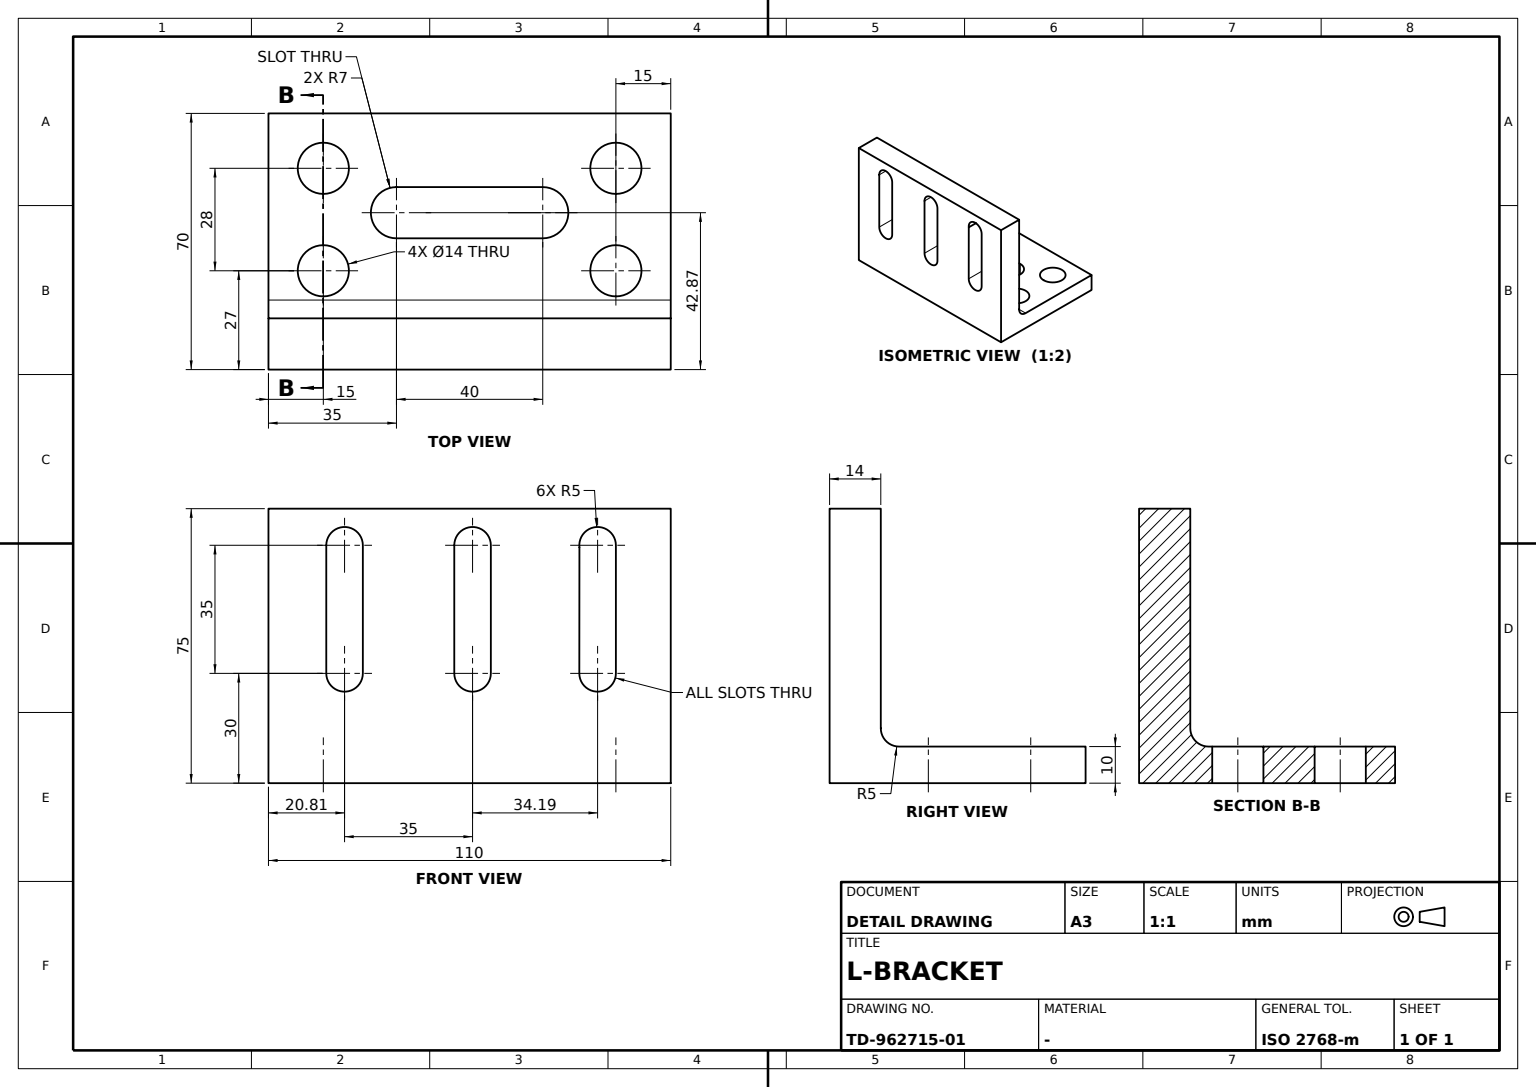
CATIA V5 part; units mm, degrees
sketch "Sketch1" plane through (0, 0, 0) normal (0, 1, 0) x (-1, 0, 0)
  line L0 (7, 54.9017) -> (7, -10.0983)
  line L1 (7, -10.0983) -> (63, -10.0983)
  line L2 (63, -10.0983) -> (63, -20.0983)
  line L3 (63, -20.0983) -> (-7, -20.0983)
  line L4 (-7, -20.0983) -> (-7, 54.9017)
  line L5 (-7, 54.9017) -> (7, 54.9017)
  dimension "length L4" = 75
  dimension "length L3" = 70
  dimension "length L5" = 14
  dimension "length L2" = 10
  constraint vertical L0 y-axis
  constraint vertical L2 y-axis
  constraint vertical L4 y-axis
  constraint horizontal L1 x-axis
  constraint horizontal L3 x-axis
  constraint horizontal L5 x-axis
  constraint symmetry L4 L0 y-axis
extrude "Pad1" add sketch "Sketch1" against normal blind 110
fillet "Fillet1" radius 5 1 edges at (-7, -55, -10.0983)
sketch "Sketch2" plane through (-7, 0, 0) normal (-1, 0, 0) x (0, -1, 0)
  arc A0 (24.9694, 44.349) -> (15, 44.9017) centre (20, 44.9017) ccw
  point P0 (20, 44.9017)
  arc A1 (59.1907, 44.9017) -> (49.1907, 44.9017) centre (54.1907, 44.9017) ccw
  point P1 (54.1907, 44.9017)
  arc A2 (94.1907, 44.9017) -> (84.1907, 44.9017) centre (89.1907, 44.9017) ccw
  point P2 (89.1907, 44.9017)
  arc A3 (15, 9.9017) -> (25, 9.9062) centre (20, 9.9017) ccw
  point P3 (20, 9.9017)
  arc A4 (49.1907, 9.9017) -> (59.1907, 9.9017) centre (54.1907, 9.9017) ccw
  point P4 (54.1907, 9.9017)
  arc A5 (84.1907, 9.9017) -> (94.1907, 9.9017) centre (89.1907, 9.9017) ccw
  point P5 (89.1907, 9.9017)
  line L0 (0, 54.9017) -> (110, 54.9017) construction
  line L1 (0, 54.9017) -> (110, 54.9017) construction
  line L2 (0, 54.9017) -> (110, 54.9017) construction
  line L3 (15, 44.9017) -> (15, 9.9017)
  line L4 (24.9694, 44.349) -> (25, 9.9062)
  line L5 (49.1907, 44.9017) -> (49.1907, 9.9017)
  line L6 (59.1907, 44.9017) -> (59.1907, 9.9017)
  line L7 (84.1907, 44.9017) -> (84.1907, 9.9017)
  line L8 (94.1907, 44.9017) -> (94.1907, 9.9017)
  point P6 (49.1907, 9.9017)
  point P7 (59.1907, 9.9017)
  point P8 (49.1907, 9.9017)
  point P9 (59.1907, 9.9017)
  line L9 (0, -10.0983) -> (0, 54.9017) construction
  dimension "radius A0" = 5
  dimension "radius A1" = 5
  dimension "radius A2" = 5
  dimension "radius A5" = 5
  dimension "radius A4" = 5
  dimension "radius A3" = 5
  dimension "distance L0 P0" = 10
  dimension "distance P2 L1" = 10
  dimension "distance L2 P1" = 10
  dimension "distance P1 P4" = 35
  dimension "distance P2 P5" = 35
  dimension "distance P0 P3" = 35
  dimension "distance L9 P0" = 20
  dimension "distance P1 P2" = 35
  constraint vertical L3 y-axis
  constraint vertical L5 y-axis
  constraint vertical L6 y-axis
  constraint vertical L7 y-axis
  constraint vertical L8 y-axis
  constraint tangency L4 A3
  constraint tangency A0 L3
  constraint tangency L5 A1
  constraint tangency L6 A1
  constraint tangency A2 L7
  constraint tangency L8 A2
  constraint coincidence A4 P6
  constraint coincidence A4 P7
  constraint coincidence L6 P9
  constraint coincidence L5 P8
  constraint coincidence P6 P8
  constraint coincidence P7 P9
extrude "Pocket1" cut sketch "Sketch2" against normal through all
sketch "Sketch3" plane through (0, 0, -10.0983) normal (0, 0, 1) x (1, 0, 0)
  arc A0 (-28.8675, -35) -> (-42.8675, -35) centre (-35.8675, -35) ccw
  point P0 (-35.8675, -35)
  arc A1 (-42.8675, -75) -> (-28.8675, -75) centre (-35.8675, -75) ccw
  point P1 (-35.8675, -75)
  line L0 (-63, -110) -> (-7, -110) construction
  line L1 (-63, 0) -> (-7, 0) construction
  line L2 (-42.8675, -35) -> (-42.8675, -75)
  line L3 (-28.8675, -35) -> (-28.8675, -75)
  circle A2 centre (-48, -15) radius 7
  point P2 (-48, -15)
  line L4 (-63, 0) -> (-63, -110) construction
  circle A3 centre (-20, -15) radius 7
  point P3 (-20, -15)
  circle A4 centre (-48, -95) radius 7
  point P4 (-48, -95)
  line L5 (-63, 0) -> (-63, -110) construction
  circle A5 centre (-20, -95) radius 7
  point P5 (-20, -95)
  line L6 (-63, -110) -> (-7, -110) construction
  line L7 (-63, 0) -> (-7, 0) construction
  line L8 (-63, -110) -> (-7, -110) construction
  line L9 (-63, 0) -> (-7, 0) construction
  dimension "radius A1" = 7
  dimension "radius A0" = 7
  dimension "distance P0 P1" = 40
  dimension "distance L0 P1" = 35
  dimension "distance L1 P0" = 35
  dimension "radius A2" = 7
  dimension "distance P2 L4" = 15
  dimension "radius A3" = 7
  dimension "distance P2 P3" = 28
  dimension "radius A4" = 7
  dimension "distance L5 P4" = 15
  dimension "radius A5" = 7
  dimension "distance P4 P5" = 28
  dimension "distance L6 P4" = 15
  dimension "distance L7 P2" = 15
  dimension "distance L8 P5" = 15
  dimension "distance L9 P3" = 15
  constraint vertical L2 y-axis
  constraint vertical L3 y-axis
  constraint tangency A0 L2
  constraint tangency L3 A0
extrude "Pocket2" cut sketch "Sketch3" against normal through all
